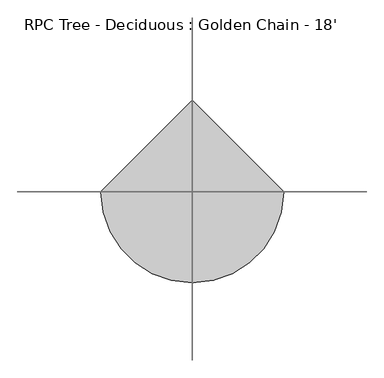
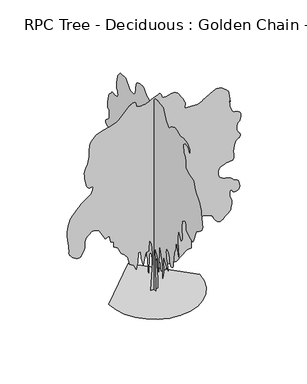
"""IFC4 building model written with IfcOpenShell, lengths in millimetres: geographic element geometry, RPC Tree - Deciduous : Golden Chain - 18'."""

from ifc_helpers import new_model, si_unit, origin, place, context, project, spatial, triangles, source, transform, mapped, element, save


def rpc_tree_deciduous_golden_chain_18_92130817(model_context):
    return source(origin(), model_context, "Body", "Tessellation", [
        triangles([(-0.0021439, 84.0442886, 0.0017013), (-0.0021439, -79.514705, 0.0017013), (-0.0021439, -54.9808464, 768.7285137), (-0.0021439, -30.4472354, 1202.1592524), (-0.0021439, -128.5824313, 1087.6687117), (-0.0021439, -161.2943336, 981.3544888), (-0.0021439, -161.2943336, 776.9073023), (-0.0021439, -202.1840252, 613.3465736), (-0.0021439, -226.7178838, 1406.6089096), (-0.0021439, -292.140671, 1251.2269695), (-0.0021439, -390.2761053, 932.2867716), (-0.0021439, -406.6337188, 556.102575), (-0.0021439, -447.5226474, 752.37348), (-0.0021439, -422.9887888, 1120.3813951), (-0.0021439, -398.4548939, 1226.6931473), (-0.0021439, -562.0131517, 1022.2459608), (-0.0021439, -643.7935524, 907.7528767), (-0.0021439, -570.1919403, 1161.2703238), (-0.0021439, -564.9696937, 1199.7284414), (-0.0021439, -559.9633495, 1237.6125389), (-0.0021439, -555.386267, 1274.3536102), (-0.0021439, -551.4518414, 1309.3777805), (-0.0021439, -548.3758664, 1342.1157532), (-0.0021439, -546.37181, 1371.9887844), (-0.0021439, -545.6580817, 1398.4301937), (-0.0021439, -546.8493608, 1421.534016), (-0.0021439, -550.1869114, 1442.0622688), (-0.0021439, -555.312616, 1460.4442863), (-0.0021439, -561.8709002, 1477.1091122), (-0.0021439, -569.5010668, 1492.488842), (-0.0021439, -577.8449615, 1507.0100487), (-0.0021439, -586.5470103, 1521.0994503), (-0.0021439, -614.3955648, 1489.5551548), (-0.0021439, -641.0985861, 1458.0134754), (-0.0021439, -665.5130842, 1426.4691799), (-0.0021439, -686.4960331, 1394.9248844), (-0.0021439, -702.8993196, 1363.383205), (-0.0021439, -713.5800631, 1331.8389095), (-0.0021439, -717.3950918, 1300.294614), (-0.0021439, -719.0638853, 1269.9442863), (-0.0021439, -723.7375099, 1241.7375778), (-0.0021439, -730.9130167, 1215.3215303), (-0.0021439, -740.0925436, 1190.333012), (-0.0021439, -750.773287, 1166.4189194), (-0.0021439, -762.4572395, 1143.2210621), (-0.0021439, -774.6391268, 1120.3813951), (-0.0021439, -797.2654346, 1120.6430071), (-0.0021439, -818.9620754, 1122.4794502), (-0.0021439, -838.7995274, 1127.4629396), (-0.0021439, -855.847978, 1137.1656904), (-0.0021439, -869.1753622, 1153.1626064), (-0.0021439, -877.8545563, 1177.0309896), (-0.0021439, -880.9533497, 1210.3380409), (-0.0021439, -882.6221432, 1252.4664288), (-0.0021439, -887.2956951, 1301.0338131), (-0.0021439, -894.4712019, 1354.9656956), (-0.0021439, -903.6508015, 1413.1900486), (-0.0021439, -914.3314722, 1474.6301937), (-0.0021439, -926.0154974, 1538.2190449), (-0.0021439, -938.1998554, 1602.8797783), (-0.0021439, -1003.6226789, 1758.2592476), (-0.0021439, -1028.1565012, 2036.3105896), (-0.0021439, -1134.4707968, 1611.0560234), (-0.0021439, -1093.5793247, 2028.1317284), (-0.0021439, -1118.113147, 2379.7846825), (-0.0021439, -1257.140126, 2134.4460239), (-0.0021439, -1267.5820759, 2148.5354256), (-0.0021439, -1277.5946915, 2163.0564869), (-0.0021439, -1286.7514, 2178.433746), (-0.0021439, -1294.6202511, 2195.1011879), (-0.0021439, -1300.7697304, 2213.4832054), (-0.0021439, -1304.7752998, 2234.0114582), (-0.0021439, -1306.2077705, 2257.1152805), (-0.0021439, -1304.3942184, 2284.415213), (-0.0021439, -1299.7206665, 2316.2921917), (-0.0021439, -1293.332539, 2351.3162167), (-0.0021439, -1286.3704639, 2388.0574333), (-0.0021439, -1279.9797203, 2425.0855511), (-0.0021439, -1275.3061684, 2460.9680992), (-0.0021439, -1273.4950871, 2494.2750778), (-0.0021439, -1274.6864388, 2526.5329926), (-0.0021439, -1278.0264965, 2560.0917), (-0.0021439, -1283.1522011, 2594.7116798), (-0.0021439, -1289.7079056, 2630.1702713), (-0.0021439, -1297.3381084, 2666.2889969), (-0.0021439, -1305.6820759, 2702.8396729), (-0.0021439, -1314.3840157, 2739.6188232), (-0.0021439, -1345.7607342, 2756.763707), (-0.0021439, -1376.1364964, 2771.6226837), (-0.0021439, -1404.5083111, 2781.8845573), (-0.0021439, -1429.8778381, 2785.2881287), (-0.0021439, -1451.239325, 2779.5474907), (-0.0021439, -1467.5969021, 2762.351738), (-0.0021439, -1477.9423462, 2731.439962), (-0.0021439, -1480.7337456, 2695.2194984), (-0.0021439, -1478.2292473, 2663.0124527), (-0.0021439, -1475.1534176, 2633.802317), (-0.0021439, -1476.2277706, 2606.5990356), (-0.0021439, -1486.169315, 2580.3861008), (-0.0021439, -1509.7024715, 2554.1987457), (-0.0021439, -1551.5464291, 2526.9879066), (-0.0021439, -1602.9255604, 2498.8777039), (-0.0021439, -1651.1601162, 2472.3397888), (-0.0021439, -1695.0995853, 2449.9522018), (-0.0021439, -1733.6059559, 2434.2878963), (-0.0021439, -1765.5313328, 2427.9227325), (-0.0021439, -1789.7298557, 2433.4293732), (-0.0021439, -1805.0613327, 2453.3862946), (-0.0021439, -1952.2644115, 2813.2027039), (-0.0021439, -2091.2889198, 2911.3481667), (-0.0021439, -2128.6269024, 2939.9231667), (-0.0021439, -2162.6730801, 2969.615831), (-0.0021439, -2192.1420662, 3000.6293449), (-0.0021439, -2215.746294, 3033.039576), (-0.0021439, -2232.1979061, 3067.0502907), (-0.0021439, -2240.209045, 3102.7626457), (-0.0021439, -2238.4919987, 3140.329248), (-0.0021439, -2229.7188423, 3187.039769), (-0.0021439, -2218.3701164, 3246.6282829), (-0.0021439, -2205.8758209, 3313.9381279), (-0.0021439, -2193.6685719, 3383.8138046), (-0.0021439, -2183.1783691, 3451.1236496), (-0.0021439, -2175.835358, 3510.7121635), (-0.0021439, -2173.0692478, 3557.3973953), (-0.0021439, -2164.9616032, 3599.7645767), (-0.0021439, -2142.2641514, 3649.0150589), (-0.0021439, -2107.4077034, 3703.9553101), (-0.0021439, -2062.820454, 3763.492955), (-0.0021439, -2010.9410625, 3826.4594604), (-0.0021439, -1954.194817, 3891.7374527), (-0.0021439, -1895.0179058, 3958.1331093), (-0.0021439, -1837.7740162, 4187.1141907), (-0.0021439, -1625.145425, 4236.1870674), (-0.0021439, -1453.4109947, 4317.9495186), (-0.0021439, -1454.7444889, 4324.4773178), (-0.0021439, -1458.0820759, 4341.9779938), (-0.0021439, -1462.4229446, 4367.5302132), (-0.0021439, -1466.7611973, 4398.0611984), (-0.0021439, -1470.0987843, 4430.6240364), (-0.0021439, -1471.4347492, 4462.1453682), (-0.0021439, -1469.7661011, 4489.7044418), (-0.0021439, -1464.1145565, 4515.6630318), (-0.0021439, -1454.6022011, 4544.1874535), (-0.0021439, -1441.8692574, 4574.8704643), (-0.0021439, -1426.5632149, 4607.280986), (-0.0021439, -1409.3241508, 4640.9614883), (-0.0021439, -1390.7999908, 4675.5308899), (-0.0021439, -1371.6305214, 4710.506662), (-0.0021439, -1338.9179832, 4906.7725891), (-0.0021439, -1445.2321335, 4996.7391907), (-0.0021439, -1576.0802513, 4972.2028976), (-0.0021439, -1649.6793926, 4865.8782829), (-0.0021439, -1649.6793926, 4964.0237457), (-0.0021439, -1535.1888519, 5070.3230713), (-0.0021439, -1347.0966991, 5094.8593643), (-0.0021439, -1199.8935476, 5062.1439194), (-0.0021439, -1052.6903961, 5143.9319504), (-0.0021439, -946.3761005, 5152.1111023), (-0.0021439, -938.5555023, 5148.3770279), (-0.0021439, -917.8620707, 5138.3694992), (-0.0021439, -888.4387213, 5123.7901566), (-0.0021439, -854.4407965, 5106.3400589), (-0.0021439, -820.0111393, 5087.7220093), (-0.0021439, -789.3025486, 5069.7132248), (-0.0021439, -766.462809, 5053.9653488), (-0.0021439, -750.6792521, 5038.3697891), (-0.0021439, -737.326506, 5021.3516418), (-0.0021439, -724.8322105, 5005.4770294), (-0.0021439, -711.6242231, 4993.3103302), (-0.0021439, -696.1277126, 4987.4426651), (-0.0021439, -676.7678478, 4990.465155), (-0.0021439, -651.9697975, 5004.8927628), (-0.0021439, -625.6020756, 5027.117569), (-0.0021439, -602.236605, 5051.5015457), (-0.0021439, -581.3730165, 5077.6383224), (-0.0021439, -562.5135209, 5105.2226852), (-0.0021439, -545.1577126, 5133.8994232), (-0.0021439, -528.8000991, 5163.2615845), (-0.0021439, -512.9454346, 5193.0051178), (-0.0021439, -414.8099639, 5397.4496155), (-0.0021439, -169.4723773, 5438.343631), (-0.0021439, -163.4401146, 5438.1913147), (-0.0021439, -147.2511773, 5437.2006775), (-0.0021439, -123.7660828, 5434.4828201), (-0.0021439, -95.8466569, 5429.1744232), (-0.0021439, -66.3536942, 5420.4621643), (-0.0021439, -38.1480076, 5407.4315643), (-0.0021439, -14.0911332, 5389.2710449), (-0.0021439, 3.3375856, 5370.932048), (-0.0021439, 15.1871941, 5356.7590759), (-0.0021439, 23.8896415, 5344.846431), (-0.0021439, 31.8767493, 5333.3907349), (-0.0021439, 41.5805652, 5320.4874527), (-0.0021439, 55.4332171, 5304.2826279), (-0.0021439, 75.8662495, 5282.9461395), (-0.0021439, 96.8951667, 5258.2575302), (-0.0021439, 112.9172356, 5234.5595581), (-0.0021439, 126.936765, 5213.8584961), (-0.0021439, 141.9573053, 5198.1611984), (-0.0021439, 160.9836875, 5189.5000992), (-0.0021439, 187.019453, 5189.8297302), (-0.0021439, 223.0691603, 5201.1836884), (-0.0021439, 263.6977487, 5220.8435349), (-0.0021439, 301.7494776, 5244.3891907), (-0.0021439, 337.654935, 5271.1352325), (-0.0021439, 371.8458713, 5300.4468155), (-0.0021439, 404.7490228, 5331.7146744), (-0.0021439, 436.7936874, 5364.2516418), (-0.0021439, 468.4065107, 5397.4496155), (-0.0021439, 491.2487575, 5406.0857162), (-0.0021439, 514.4465784, 5413.9090759), (-0.0021439, 538.360671, 5420.1825302), (-0.0021439, 563.3491894, 5424.0945007), (-0.0021439, 589.7652005, 5424.8560822), (-0.0021439, 617.9718727, 5421.6812759), (-0.0021439, 648.3223457, 5413.807338), (-0.0021439, 679.72181, 5404.5108124), (-0.0021439, 710.2653671, 5396.4845581), (-0.0021439, 739.0892618, 5388.0513519), (-0.0021439, 765.3401304, 5377.4595566), (-0.0021439, 788.156979, 5363.0069504), (-0.0021439, 806.6837551, 5342.991893), (-0.0021439, 820.0593922, 5315.6615845), (-0.0021439, 829.6199278, 5284.3687271), (-0.0021439, 837.4634897, 5253.4822403), (-0.0021439, 843.8769791, 5222.9771255), (-0.0021439, 849.1474422, 5192.7254837), (-0.0021439, 853.5569115, 5162.7284775), (-0.0021439, 857.3973747, 5132.8326279), (-0.0021439, 860.9483208, 5103.0379349), (-0.0021439, 866.3610718, 5073.4217194), (-0.0021439, 872.7034172, 5044.897879), (-0.0021439, 880.9050968, 5018.507048), (-0.0021439, 891.895705, 4995.3166031), (-0.0021439, 906.6073797, 4976.4444992), (-0.0021439, 925.9672445, 4962.9063721), (-0.0021439, 950.90751, 4955.8451752), (-0.0021439, 981.1385862, 4952.5180527), (-0.0021439, 1014.5192522, 4950.3588821), (-0.0021439, 1049.1851595, 4950.4606201), (-0.0021439, 1083.27959, 4954.016217), (-0.0021439, 1114.9432823, 4962.1442093), (-0.0021439, 1142.314286, 4976.0125488), (-0.0021439, 1163.533485, 4996.7391907), (-0.0021439, 1185.0142233, 5025.1618744), (-0.0021439, 1212.2201935, 5059.0452713), (-0.0021439, 1241.8544312, 5094.7832062), (-0.0021439, 1270.6326164, 5128.8195007), (-0.0021439, 1295.2629444, 5157.546817), (-0.0021439, 1312.4536102, 5177.4095581), (-0.0021439, 1318.9129543, 5184.8259659), (-0.0021439, 1572.4303288, 5168.4688248), (-0.0021439, 1670.5657631, 5045.7867783), (-0.0021439, 1675.8337555, 5036.8204651), (-0.0021439, 1681.1752899, 5026.6606201), (-0.0021439, 1686.6592575, 5014.0363907), (-0.0021439, 1692.3589096, 4997.7804062), (-0.0021439, 1698.3406666, 4976.6479752), (-0.0021439, 1704.683012, 4949.4444031), (-0.0021439, 1711.4546917, 4914.9511597), (-0.0021439, 1717.9875778, 4876.8767395), (-0.0021439, 1723.6619408, 4839.6656387), (-0.0021439, 1728.6225391, 4803.1402519), (-0.0021439, 1733.00919, 4767.2247116), (-0.0021439, 1736.9665066, 4731.7155418), (-0.0021439, 1740.6392475, 4696.5112953), (-0.0021439, 1744.1673752, 4661.4337852), (-0.0021439, 1726.808987, 4636.8466232), (-0.0021439, 1710.4538807, 4611.9798271), (-0.0021439, 1696.1003963, 4586.5546349), (-0.0021439, 1684.7516705, 4560.2402527), (-0.0021439, 1677.408514, 4532.8082062), (-0.0021439, 1675.0717381, 4503.9282829), (-0.0021439, 1678.7446243, 4473.3467194), (-0.0021439, 1687.7336105, 4446.5242287), (-0.0021439, 1700.5834076, 4427.9823372), (-0.0021439, 1717.1544891, 4416.0444031), (-0.0021439, 1737.3016605, 4408.9576263), (-0.0021439, 1760.8805992, 4405.0206573), (-0.0021439, 1787.7511974, 4402.5315651), (-0.0021439, 1817.7689873, 4399.7375496), (-0.0021439, 1846.9991798, 4399.6105225), (-0.0021439, 1872.3687069, 4403.8015457), (-0.0021439, 1895.0179058, 4408.5259666), (-0.0021439, 1916.094817, 4410.1261597), (-0.0021439, 1936.7425392, 4404.8683411), (-0.0021439, 1958.1038807, 4389.0187271), (-0.0021439, 1981.3271725, 4358.8435341), (-0.0021439, 2004.8831474, 4328.2872597), (-0.0021439, 2026.5797882, 4309.5930519), (-0.0021439, 2046.5593826, 4296.6136116), (-0.0021439, 2064.9668346, 4283.2278008), (-0.0021439, 2081.9416706, 4263.2380325), (-0.0021439, 2097.6312653, 4230.5228783), (-0.0021439, 2112.1752903, 4178.9353294), (-0.0021439, 2125.1928097, 4121.9123566), (-0.0021439, 2136.208707, 4075.3541519), (-0.0021439, 2145.220657, 4036.6698853), (-0.0021439, 2152.2311302, 4003.269017), (-0.0021439, 2157.2373653, 3972.5857155), (-0.0021439, 2160.239653, 3942.0294411), (-0.0021439, 2161.2429348, 3909.0602325), (-0.0021439, 2158.6191124, 3878.529538), (-0.0021439, 2151.2761013, 3856.1774139), (-0.0021439, 2139.9984467, 3840.6074341), (-0.0021439, 2125.5737457, 3830.4725876), (-0.0021439, 2108.7894505, 3824.4276077), (-0.0021439, 2090.4303967, 3821.0746147), (-0.0021439, 2071.2837456, 3819.093631), (-0.0021439, 2071.2837456, 3606.4699814), (-0.0021439, 2071.4514679, 3602.8379356), (-0.0021439, 2072.6198559, 3598.3167), (-0.0021439, 2075.7897205, 3592.093824), (-0.0021439, 2081.9671051, 3583.305407), (-0.0021439, 2092.1472977, 3571.0625496), (-0.0021439, 2107.334016, 3554.5525108), (-0.0021439, 2128.5303967, 3532.8863914), (-0.0021439, 2153.3512653, 3510.1278969), (-0.0021439, 2177.8850876, 3490.1125488), (-0.0021439, 2200.8441513, 3471.4944992), (-0.0021439, 2220.9432152, 3453.054055), (-0.0021439, 2236.8944218, 3433.4453682), (-0.0021439, 2247.4099136, 3411.4234566), (-0.0021439, 2251.1996532, 3385.6677612), (-0.0021439, 2244.7632729, 3361.4363914), (-0.0021439, 2226.7369022, 3344.0880318), (-0.0021439, 2199.0560337, 3332.4547302), (-0.0021439, 2163.6509274, 3325.3935333), (-0.0021439, 2122.4495178, 3321.7614876), (-0.0021439, 2077.3874428, 3320.440638), (-0.0021439, 2030.394817, 3320.2374527), (-0.0021439, 2016.5671726, 3321.7614876), (-0.0021439, 2003.8823364, 3321.9393837), (-0.0021439, 1993.4861687, 3319.3991318), (-0.0021439, 1986.5265644, 3312.7698853), (-0.0021439, 1984.1415356, 3300.704924), (-0.0021439, 1987.4789772, 3281.8325294), (-0.0021439, 1997.6847496, 3254.8324333), (-0.0021439, 2015.3987846, 3226.9687271), (-0.0021439, 2039.2646244, 3205.2770279), (-0.0021439, 2067.4229347, 3187.8780899), (-0.0021439, 2098.0122013, 3172.892086), (-0.0021439, 2129.1729446, 3158.4903488), (-0.0021439, 2159.0484467, 3142.8183403), (-0.0021439, 2185.7769024, 3123.9715256), (-0.0021439, 2209.1905895, 3107.7664101), (-0.0021439, 2229.8839485, 3098.4193062), (-0.0021439, 2247.1458309, 3091.789769), (-0.0021439, 2260.259856, 3083.7379349), (-0.0021439, 2268.5097885, 3070.0983604), (-0.0021439, 2271.1792477, 3046.7303101), (-0.0021439, 2267.5547596, 3009.4939201), (-0.0021439, 2258.1617283, 2968.2188232), (-0.0021439, 2244.4762264, 2934.6653481), (-0.0021439, 2227.2144894, 2907.5635139), (-0.0021439, 2207.0926071, 2885.592762), (-0.0021439, 2184.8218735, 2867.5078194), (-0.0021439, 2161.1236107, 2851.9884178), (-0.0021439, 2136.7091125, 2837.7389969), (-0.0021439, 2128.1010624, 2820.1877426), (-0.0021439, 2120.4252228, 2802.3315651), (-0.0021439, 2114.6061012, 2783.8911209), (-0.0021439, 2111.5783791, 2764.6123558), (-0.0021439, 2112.2691799, 2744.1653481), (-0.0021439, 2117.6108597, 2722.2960434), (-0.0021439, 2128.5303967, 2698.7248077), (-0.0021439, 2148.3677032, 2676.3473946), (-0.0021439, 2177.0748173, 2656.8148659), (-0.0021439, 2210.5012653, 2637.9933403), (-0.0021439, 2244.4991901, 2617.7495178), (-0.0021439, 2274.9232052, 2593.9245186), (-0.0021439, 2297.620657, 2564.3841705), (-0.0021439, 2308.446159, 2526.9879066), (-0.0021439, 2310.9024044, 2485.6212456), (-0.0021439, 2311.0675106, 2444.3970177), (-0.0021439, 2308.6595181, 2401.4558887), (-0.0021439, 2303.3915257, 2354.9408501), (-0.0021439, 2294.9740162, 2302.9877712), (-0.0021439, 2283.1248848, 2243.7396435), (-0.0021439, 2267.5547596, 2175.3349525), (-0.0021439, 2251.3672302, 2117.0648174), (-0.0021439, 2237.1813229, 2082.6833405), (-0.0021439, 2223.9962265, 2062.0356182), (-0.0021439, 2210.8111301, 2044.9642765), (-0.0021439, 2196.6252228, 2021.3144119), (-0.0021439, 2180.4352226, 1980.9232727), (-0.0021439, 2161.2429348, 1913.6411877), (-0.0021439, 2144.2656281, 1837.9644115), (-0.0021439, 2133.5848846, 1778.8840061), (-0.0021439, 2126.4805218, 1735.9681664), (-0.0021439, 2120.2346821, 1708.7877033), (-0.0021439, 2112.1270374, 1696.9131374), (-0.0021439, 2099.4422012, 1699.9180412), (-0.0021439, 2079.4626068, 1717.370319), (-0.0021439, 2055.4062263, 1753.7304543), (-0.0021439, 2032.2085144, 1808.9728672), (-0.0021439, 2009.7244217, 1875.9475582), (-0.0021439, 1987.8118057, 1947.4968246), (-0.0021439, 1966.3309948, 2016.4731377), (-0.0021439, 1945.1347595, 2075.7211201), (-0.0021439, 1924.0831375, 2118.0884468), (-0.0021439, 1898.5232151, 2149.1551552), (-0.0021439, 1864.8097206, 2179.3659565), (-0.0021439, 1824.3018734, 2208.8579063), (-0.0021439, 1778.3583115, 2237.7782341), (-0.0021439, 1728.3354927, 2266.2695183), (-0.0021439, 1675.5974327, 2294.4762268), (-0.0021439, 1621.4979733, 2322.5380314), (-0.0021439, 1576.1971046, 2351.8395859), (-0.0021439, 1532.4709946, 2378.2097786), (-0.0021439, 1491.8919308, 2398.715213), (-0.0021439, 1456.032201, 2410.4220566), (-0.0021439, 1426.4667091, 2410.3966221), (-0.0021439, 1404.769923, 2395.7104546), (-0.0021439, 1392.5144211, 2363.42696), (-0.0021439, 1384.3127415, 2321.608437), (-0.0021439, 1373.9674427, 2280.2191029), (-0.0021439, 1361.8312649, 2239.1854156), (-0.0021439, 1348.2650871, 2198.4387749), (-0.0021439, 1333.6245564, 2157.9054932), (-0.0021439, 1318.270261, 2117.5168247), (-0.0021439, 1302.557848, 2077.1995182), (-0.0021439, 1122.642013, 1921.8200489), (-0.0021439, 1105.2379154, 1902.4119312), (-0.0021439, 1088.5475824, 1882.2163616), (-0.0021439, 1073.2897928, 1860.4485043), (-0.0021439, 1060.1757677, 1836.3210526), (-0.0021439, 1049.9243586, 1809.0440838), (-0.0021439, 1043.2491846, 1777.8350876), (-0.0021439, 1040.8641558, 1741.9041412), (-0.0021439, 1040.1478477, 1706.9283691), (-0.0021439, 1038.1463711, 1678.3863613), (-0.0021439, 1035.070396, 1655.2139385), (-0.0021439, 1031.1359705, 1636.3290447), (-0.0021439, 1026.5588516, 1620.6648846), (-0.0021439, 1021.5525438, 1607.1469597), (-0.0021439, 1016.3302608, 1594.7010624), (-0.0021439, 869.1271093, 1496.5656281), (-0.0021439, 852.7720757, 1324.8285816), (-0.0021439, 730.1027464, 1267.5820759), (-0.0021439, 697.3900629, 1054.9560282), (-0.0021439, 566.5419814, 1022.2459608), (-0.0021439, 578.5586898, 1016.8332098), (-0.0021439, 589.0742907, 1010.4907917), (-0.0021439, 596.5850967, 1002.2891848), (-0.0021439, 599.5873844, 991.2985765), (-0.0021439, 596.5850967, 976.5869019), (-0.0021439, 586.0694959, 957.227037), (-0.0021439, 566.5419814, 932.2867716), (-0.0021439, 542.9631517, 906.6327415), (-0.0021439, 521.098825, 885.268784), (-0.0021439, 500.6670779, 867.4837503), (-0.0021439, 481.3782844, 852.5587166), (-0.0021439, 462.9480503, 839.7799181), (-0.0021439, 445.0893293, 828.4287214), (-0.0021439, 427.5175821, 817.7962309), (-0.0021439, 415.2874784, 850.3895176), (-0.0021439, 403.27077, 878.7613323), (-0.0021439, 391.6832869, 898.6927465), (-0.0021439, 380.7384244, 905.9647591), (-0.0021439, 370.6545922, 896.3558979), (-0.0021439, 361.6401352, 865.6473072), (-0.0021439, 353.9160064, 809.6174423), (-0.0021439, 346.4306348, 755.6856325), (-0.0021439, 338.0841966, 726.6457626), (-0.0021439, 329.0239938, 711.3397928), (-0.0021439, 319.3923142, 698.6092472), (-0.0021439, 309.3313731, 677.2936152), (-0.0021439, 298.9834219, 636.2370369), (-0.0021439, 288.4932192, 564.2788201), (-0.0021439, 279.4076364, 484.1215035), (-0.0021439, 272.9001666, 423.7050605), (-0.0021439, 268.5364431, 379.7401932), (-0.0021439, 265.889766, 348.9350604), (-0.0021439, 264.5308555, 328.0029442), (-0.0021439, 264.0304863, 313.6493872), (-0.0021439, 263.9593606, 302.5851461), (-0.0021439, 239.4252477, 809.6174423), (-0.0021439, 227.0988743, 842.5688467), (-0.0021439, 214.4146195, 873.4450871), (-0.0021439, 201.0151103, 900.1709993), (-0.0021439, 186.5429559, 920.6764338), (-0.0021439, 170.6400022, 932.8836828), (-0.0021439, 152.9489127, 934.7200533), (-0.0021439, 133.1120149, 924.1105265), (-0.0021439, 115.4209072, 902.0556953), (-0.0021439, 103.7379267, 871.8474375), (-0.0021439, 97.0620442, 834.8447542), (-0.0021439, 94.3917403, 792.4038855), (-0.0021439, 94.7254953, 745.8888468), (-0.0021439, 97.0620442, 696.65348), (-0.0021439, 100.3998583, 646.0591845), (-0.0021439, 84.0442886, 237.1621046), (88.2248747, 0.0002499, 0.0), (-86.1796688, 0.0002499, 0.0), (-44.6549823, 0.000202, 805.5838949), (-36.3499433, 0.0001914, 1029.8176643), (-69.5698451, 0.0001754, 1303.8836391), (-127.7051138, 0.0001648, 1445.0670273), (-144.3149375, 0.0001861, 1137.7829493), (-227.3643014, 0.0001861, 1112.8680456), (-293.8043594, 0.000202, 797.2781519), (-351.9398915, 0.0001914, 996.5995611), (-360.2456709, 0.0001808, 1179.3068682), (-426.6844571, 0.0001808, 1179.3068682), (-443.2935451, 0.0001967, 913.5491798), (-484.8200074, 0.0002073, 730.8393293), (-551.2587936, 0.000202, 872.0227175), (-659.2240059, 0.0001967, 938.4640108), (-700.7479248, 0.0001808, 1154.3919645), (-783.7983788, 0.0001754, 1254.0539772), (-875.1545031, 0.0001754, 1328.7985428), (-974.8139723, 0.0001595, 1519.8115929), (-1082.7792572, 0.0001595, 1577.9471432), (-1082.7792572, 0.0001489, 1719.1331474), (-1157.5238228, 0.0001489, 1744.0479057), (-1199.0477417, 0.0001382, 1935.0611012), (-1315.3188423, 0.0001382, 1885.2312939), (-1464.8079735, 0.0001223, 2167.6005409), (-1498.6102707, 0.0001223, 2188.6191708), (-1532.3364098, 0.0001223, 2207.6005703), (-1565.920261, 0.000117, 2222.5153576), (-1599.2856663, 0.000117, 2231.3292091), (-1632.3590836, 0.000117, 2232.0073654), (-1665.071767, 0.000117, 2222.5153576), (-1697.3475586, 0.0001223, 2200.8213329), (-1729.1864582, 0.0001223, 2173.6305508), (-1759.8645275, 0.0001223, 2148.0374908), (-1788.2186108, 0.0001276, 2122.5893349), (-1813.0851162, 0.0001276, 2095.8354446), (-1833.3035042, 0.0001276, 2066.3206764), (-1847.7078575, 0.0001329, 2032.5919212), (-1855.1424328, 0.0001329, 1993.1966515), (-1857.4665642, 0.0001382, 1950.0978287), (-1858.4826359, 0.0001382, 1906.709634), (-1859.9354542, 0.0001435, 1863.7555698), (-1863.5676453, 0.0001435, 1821.9649521), (-1871.12169, 0.0001435, 1782.0615738), (-1884.3423946, 0.0001489, 1744.7744602), (-1904.9722401, 0.0001489, 1710.8272591), (-1925.8916027, 0.0001542, 1679.5447208), (-1941.1469215, 0.0001542, 1650.7309273), (-1954.2202515, 0.0001542, 1625.8414581), (-1968.6042572, 0.0001542, 1606.3240448), (-1987.7812843, 0.0001595, 1593.6367378), (-2015.2387653, 0.0001595, 1589.2298847), (-2054.4613712, 0.0001595, 1594.5563038), (-2100.8772881, 0.0001542, 1610.4896336), (-2146.1325199, 0.0001542, 1635.5747303), (-2188.0426071, 0.0001542, 1667.7768345), (-2224.4355892, 0.0001489, 1705.0640934), (-2253.1274426, 0.0001489, 1745.4043636), (-2271.9412651, 0.0001435, 1786.7580894), (-2278.6952133, 0.0001435, 1827.0983597), (-2278.3572979, 0.0001435, 1862.6177032), (-2278.0195278, 0.0001382, 1894.6496143), (-2278.6952133, 0.0001382, 1928.8635143), (-2281.4078384, 0.0001329, 1970.9208309), (-2287.1711494, 0.0001329, 2026.4883694), (-2297.0009274, 0.0001276, 2101.2355511), (-2311.91586, 0.0001223, 2200.8213329), (-2322.6194218, 0.0001116, 2312.733688), (-2321.2629639, 0.0001063, 2418.8346245), (-2311.0445469, 0.000101, 2516.3629738), (-2295.1619408, 9.57e-05, 2602.5603287), (-2276.8079739, 9.04e-05, 2674.6710434), (-2259.1802708, 9.04e-05, 2729.9159271), (-2245.4770374, 8.51e-05, 2765.552124), (-2223.2494698, 8.51e-05, 2800.0962364), (-2182.5714294, 7.97e-05, 2849.5754837), (-2130.4174908, 7.97e-05, 2907.6399628), (-2073.7603386, 7.44e-05, 2967.8886108), (-2019.5719311, 7.44e-05, 3023.9209465), (-1974.8248077, 6.91e-05, 3069.3361977), (-1946.496159, 6.91e-05, 3097.7588814), (-1919.5238228, 6.38e-05, 3119.3488426), (-1878.1676262, 6.38e-05, 3147.4921829), (-1828.3860718, 6.38e-05, 3180.5628387), (-1776.1357727, 5.85e-05, 3216.9864876), (-1727.37029, 5.85e-05, 3255.1373566), (-1688.0485622, 5.32e-05, 3293.4405418), (-1664.1269119, 5.32e-05, 3330.2958504), (-1652.0695084, 5.32e-05, 3362.9857155), (-1643.9338131, 4.78e-05, 3390.4430511), (-1639.0672497, 4.78e-05, 3413.5317581), (-1636.8141895, 4.78e-05, 3433.1657341), (-1636.5246723, 4.78e-05, 3450.1585922), (-1637.5405987, 4.78e-05, 3465.3983597), (-1639.2120083, 4.25e-05, 3479.8003876), (-1669.3566799, 4.25e-05, 3474.8727814), (-1698.8486298, 4.25e-05, 3472.5104256), (-1727.0325199, 4.25e-05, 3475.2029938), (-1753.2554832, 4.25e-05, 3485.5407349), (-1776.8621819, 4.25e-05, 3506.0639008), (-1797.2025101, 4.25e-05, 3539.2871635), (-1813.6185139, 3.72e-05, 3587.7501938), (-1828.0965546, 3.19e-05, 3649.192955), (-1841.9954155, 3.19e-05, 3717.1379356), (-1853.7124329, 2.66e-05, 3788.029248), (-1861.6551167, 2.13e-05, 3858.1586884), (-1864.2229832, 1.59e-05, 3923.9447891), (-1859.8161301, 1.59e-05, 3981.7552139), (-1846.8366898, 1.06e-05, 4027.907048), (-1827.3218925, 1.06e-05, 4070.527993), (-1805.6277225, 5.3e-06, 4119.6770279), (-1783.6414192, 5.3e-06, 4174.7951752), (-1763.2554543, 0.0, 4235.2725883), (-1746.3543056, -5.3e-06, 4300.5505806), (-1734.827829, -1.06e-05, 4370.0448853), (-1730.5682053, -1.06e-05, 4443.1715263), (-1731.1981087, -1.59e-05, 4512.6914108), (-1731.5358788, -2.13e-05, 4573.1941132), (-1729.2601456, -2.13e-05, 4626.8643837), (-1722.0438709, -2.66e-05, 4675.9116806), (-1707.5659756, -3.19e-05, 4722.4698853), (-1683.4969505, -3.19e-05, 4768.7234573), (-1647.5177513, -3.72e-05, 4816.881855), (-1600.690377, -3.72e-05, 4863.1860054), (-1547.4697884, -4.25e-05, 4902.5054077), (-1490.6194794, -4.25e-05, 4934.9917969), (-1432.8953865, -4.25e-05, 4960.8233597), (-1377.0611492, -4.25e-05, 4980.0768356), (-1325.8750294, -4.78e-05, 4992.9801178), (-1282.0980503, -4.78e-05, 4999.6093643), (-1235.7558208, -4.78e-05, 5007.4071442), (-1178.8064627, -4.78e-05, 5022.3172806), (-1116.9168537, -4.78e-05, 5042.3067581), (-1055.7561974, -4.78e-05, 5065.3698853), (-1000.9861393, -5.32e-05, 5089.4236496), (-958.2760283, -5.32e-05, 5112.4867767), (-933.2875099, -5.32e-05, 5132.4768356), (-667.5298216, -6.91e-05, 5414.8485535), (-644.4056517, -6.91e-05, 5430.6981674), (-621.3551691, -7.44e-05, 5445.4304077), (-598.4494452, -7.44e-05, 5458.0034775), (-575.7621672, -7.44e-05, 5467.2994217), (-553.3669862, -7.44e-05, 5472.2270279), (-531.3324663, -7.44e-05, 5471.7195007), (-509.7348747, -7.44e-05, 5464.6833023), (-494.6015325, -7.44e-05, 5448.9860046), (-488.3302946, -6.91e-05, 5425.5926651), (-485.5464529, -6.91e-05, 5398.0083023), (-480.8728283, -6.91e-05, 5369.6617767), (-468.9348215, -6.91e-05, 5344.109848), (-444.3603404, -6.38e-05, 5324.7802139), (-401.7696261, -6.38e-05, 5315.1790558), (-351.2845536, -6.38e-05, 5313.8076279), (-306.0319379, -6.38e-05, 5316.3475891), (-265.1379224, -6.38e-05, 5322.1640945), (-227.7280329, -6.38e-05, 5330.5967194), (-192.9340992, -6.38e-05, 5340.9856201), (-159.8838637, -6.91e-05, 5352.6692093), (-127.7051138, -6.91e-05, 5365.0138046), (-76.3011021, -6.91e-05, 5394.9858124), (-26.1320305, -6.91e-05, 5423.3067581), (21.5672178, -7.44e-05, 5448.2750015), (65.5619775, -7.44e-05, 5468.2139008), (104.6172789, -7.44e-05, 5481.4729752), (137.4980844, -7.44e-05, 5486.4005814), (162.9699762, -7.44e-05, 5481.295079), (179.3133463, -7.44e-05, 5468.6964294), (187.9572228, -7.44e-05, 5452.7706573), (192.3880025, -7.44e-05, 5434.2287659), (196.092591, -6.91e-05, 5413.7817581), (202.5574036, -6.91e-05, 5392.1917969), (215.2690732, -6.91e-05, 5370.1448868), (237.7143056, -6.91e-05, 5348.4020279), (275.0261451, -6.38e-05, 5338.7758713), (326.72021, -6.91e-05, 5346.5736511), (387.858048, -6.91e-05, 5362.8040558), (453.4992448, -6.91e-05, 5378.4251953), (518.703586, -6.91e-05, 5384.495755), (578.5332916, -6.91e-05, 5371.9482651), (628.0480745, -6.38e-05, 5331.7908325), (667.8549471, -6.38e-05, 5276.5453674), (702.431979, -5.85e-05, 5224.3485535), (732.6477945, -5.85e-05, 5174.6917007), (759.3787937, -5.32e-05, 5127.0667007), (783.4960716, -5.32e-05, 5080.9654449), (805.8683979, -4.78e-05, 5035.8804062), (827.3694838, -4.78e-05, 4991.303476), (819.0637407, -3.72e-05, 4841.7992294), (1101.4329878, -3.72e-05, 4825.1874527), (1128.1156614, -3.72e-05, 4827.1178581), (1154.7247204, -3.72e-05, 4829.8104263), (1181.1890207, -3.72e-05, 4834.1284767), (1207.4373459, -3.72e-05, 4840.8338814), (1233.3936104, -3.72e-05, 4850.7399628), (1258.9866703, -3.72e-05, 4864.6338821), (1284.1428383, -3.72e-05, 4883.3280899), (1314.3840157, -4.25e-05, 4906.391217), (1354.2163227, -4.25e-05, 4932.4774155), (1402.0343342, -4.25e-05, 4961.1285736), (1456.2481762, -4.78e-05, 4991.8115845), (1515.2548943, -4.78e-05, 5024.0189209), (1577.4569115, -4.78e-05, 5057.2168945), (1641.2566509, -5.32e-05, 5090.9479752), (1680.2888615, -5.32e-05, 5087.2394806), (1718.5920467, -5.32e-05, 5082.6676666), (1755.4448845, -5.32e-05, 5076.3680511), (1790.1184948, -4.78e-05, 5067.4273178), (1821.883707, -4.78e-05, 5055.0065643), (1850.0193443, -4.78e-05, 5038.2174728), (1873.796236, -4.78e-05, 5016.2211411), (1895.5158405, -4.78e-05, 4994.8090759), (1917.3800583, -4.25e-05, 4978.1972992), (1938.5180122, -4.25e-05, 4963.0331085), (1958.0582439, -4.25e-05, 4945.9899628), (1975.1269695, -4.25e-05, 4923.7139969), (1988.8557827, -3.72e-05, 4892.8786697), (1998.3730797, -3.72e-05, 4850.1051178), (2031.5912556, -2.13e-05, 4609.2622604), (2026.3130894, -2.66e-05, 4631.7411209), (2021.3982731, -2.66e-05, 4650.2068542), (2017.2097206, -2.66e-05, 4660.6972023), (2014.1109272, -2.66e-05, 4659.1984566), (2012.4624813, -2.66e-05, 4641.7233604), (2012.6326744, -2.13e-05, 4604.2584961), (2014.982095, -2.13e-05, 4542.8157349), (2024.0372108, -1.59e-05, 4472.7371635), (2041.6649139, -1.06e-05, 4412.2344612), (2064.2302517, -5.3e-06, 4361.7392876), (2088.1036491, -5.3e-06, 4321.7088821), (2109.6530605, -5.3e-06, 4292.6004845), (2125.2461494, -5.3e-06, 4274.7948853), (2131.2507248, 0.0, 4268.7751945), (2142.2438038, 0.0, 4269.5626465), (2170.3794411, 0.0, 4269.054538), (2208.3929638, 0.0, 4262.8822403), (2249.0228966, 0.0, 4246.6771248), (2285.0019505, 0.0, 4216.0955612), (2309.0709755, 5.3e-06, 4166.7686302), (2313.9605026, 1.06e-05, 4094.3532829), (2302.3145565, 1.06e-05, 4025.0874527), (2283.8411201, 1.59e-05, 3981.5264488), (2261.8803967, 1.59e-05, 3953.8150589), (2239.7721531, 1.59e-05, 3932.0472015), (2220.8644409, 2.13e-05, 3906.3423752), (2208.4894695, 2.13e-05, 3866.8453674), (2205.9977612, 2.66e-05, 3803.6756767), (2214.1080219, 2.66e-05, 3738.0166031), (2229.1931477, 3.19e-05, 3693.2617767), (2248.052607, 3.19e-05, 3662.9089783), (2267.4963329, 3.72e-05, 3640.404538), (2284.3237942, 3.72e-05, 3619.1700783), (2295.3423077, 3.72e-05, 3592.7539581), (2297.3514874, 4.25e-05, 3554.5272217), (2288.6113232, 4.25e-05, 3520.3133217), (2271.1538132, 4.25e-05, 3503.5492287), (2247.4479927, 4.25e-05, 3494.176545), (2219.9678387, 4.25e-05, 3482.1877419), (2191.1768635, 4.78e-05, 3457.5500015), (2163.5518055, 4.78e-05, 3410.2805031), (2139.5564678, 5.32e-05, 3330.2958504), (2124.616246, 5.85e-05, 3235.8585915), (2119.7039005, 6.38e-05, 3152.4703674), (2120.5978867, 6.91e-05, 3080.9947884), (2123.0922112, 7.44e-05, 3022.3207535), (2122.9702709, 7.44e-05, 2977.2865837), (2116.0208405, 7.44e-05, 2946.7811783), (2098.0325489, 7.97e-05, 2931.6681473), (2075.2233307, 7.97e-05, 2926.3088814), (2054.8856186, 7.97e-05, 2923.4387077), (2034.4005318, 7.97e-05, 2921.4065643), (2011.1568924, 7.97e-05, 2918.688707), (1982.5362556, 7.97e-05, 2913.6343643), (1945.927153, 7.97e-05, 2904.642762), (1898.7111397, 7.97e-05, 2890.1392868), (1848.9295853, 7.97e-05, 2873.0196922), (1806.557317, 7.97e-05, 2855.9000977), (1771.8863228, 8.51e-05, 2836.7483597), (1745.2036491, 8.51e-05, 2813.5329163), (1726.8014294, 8.51e-05, 2784.1957535), (1716.9715061, 9.04e-05, 2746.7561783), (1716.0038326, 9.04e-05, 2699.1311783), (1719.3693249, 9.57e-05, 2651.9381287), (1723.6059849, 9.57e-05, 2615.4889), (1730.6011974, 9.57e-05, 2587.3202705), (1742.2496143, 0.000101, 2564.9937263), (1760.4309174, 0.000101, 2545.9693062), (1787.0425198, 0.000101, 2527.8387268), (1823.9665741, 0.000101, 2508.1053383), (1868.3733112, 0.000101, 2489.8733116), (1914.8146626, 0.0001063, 2476.1444984), (1961.2535431, 0.0001063, 2464.3056862), (2005.6604256, 0.0001063, 2451.7378487), (2045.9980797, 0.0001063, 2435.8296627), (2080.234798, 0.0001063, 2413.9679157), (2106.3358212, 0.0001116, 2383.5311108), (2130.3794117, 0.0001116, 2355.9518349), (2158.3448559, 0.0001116, 2339.8507828), (2188.0552517, 0.0001116, 2328.3978481), (2217.3287556, 0.0001116, 2314.7681568), (2243.9859947, 0.000117, 2292.1266609), (2265.8503578, 0.000117, 2253.6532825), (2280.7423267, 0.0001223, 2192.5154446), (2284.6387459, 0.0001276, 2127.6997787), (2276.3354736, 0.0001276, 2080.7503189), (2257.8595665, 0.0001276, 2048.6929733), (2231.2504349, 0.0001329, 2028.5482727), (2198.5377514, 0.0001329, 2017.3367477), (2161.758601, 0.0001329, 2012.084016), (2122.9474525, 0.0001329, 2009.8056667), (2101.7129929, 0.0001329, 2041.1618923), (2081.2050877, 0.0001276, 2068.4491802), (2062.1473846, 0.0001276, 2087.6032436), (2045.2716705, 0.0001276, 2094.5502033), (2031.301593, 0.0001276, 2085.2283886), (2020.9613811, 0.0001276, 2055.5688618), (2014.982095, 0.0001329, 2001.5023945), (2017.3316608, 0.0001382, 1943.077327), (2028.6854736, 0.0001382, 1899.1784077), (2044.8347786, 0.0001435, 1863.9969795), (2061.5657341, 0.0001435, 1831.721188), (2074.6671146, 0.0001435, 1796.5396145), (2079.9198463, 0.0001489, 1752.6433113), (2073.1151745, 0.0001489, 1694.2182438), (2060.9612652, 0.0001542, 1634.6526936), (2051.1314873, 0.0001595, 1588.8921146), (2040.8648174, 0.0001595, 1553.4438423), (2027.4027031, 0.0001595, 1524.8256763), (2007.9844116, 0.0001648, 1499.5475681), (1979.8489197, 0.0001648, 1474.1220852), (1940.2375294, 0.0001648, 1445.0670273), (1897.6468151, 0.0001701, 1411.1936588), (1860.8676647, 0.0001701, 1376.4489773), (1827.5758015, 0.0001701, 1345.0443535), (1795.4449139, 0.0001754, 1321.1937744), (1762.1530506, 0.0001754, 1309.1135525), (1725.3739002, 0.0001754, 1313.0099716), (1682.783186, 0.0001701, 1337.101815), (1643.0500008, 0.0001701, 1374.8030022), (1614.0660141, 0.0001701, 1414.9706085), (1592.3464096, 0.0001648, 1454.995927), (1574.4063709, 0.0001648, 1492.2577515), (1556.7559948, 0.0001595, 1524.1473747), (1535.9077034, 0.0001595, 1548.0437359), (1508.376535, 0.0001595, 1561.3381279), (1468.1125683, 0.0001595, 1573.6367958), (1415.0620274, 0.0001595, 1592.6208115), (1354.7472496, 0.0001542, 1612.7655121), (1292.689991, 0.0001542, 1628.5516125), (1234.4096821, 0.0001542, 1634.4596821), (1185.4282242, 0.0001542, 1624.9676743), (1151.2627224, 0.0001595, 1594.5563038), (1124.6054106, 0.0001595, 1573.5402901), (1095.6214966, 0.0001595, 1585.0667667), (1066.0584028, 0.0001542, 1612.8620178), (1037.6561394, 0.0001542, 1640.6597397), (1012.1621286, 0.0001542, 1652.1837456), (991.3138372, 0.0001542, 1631.1678772), (976.8586876, 0.0001595, 1561.3381279), (969.4749086, 0.0001648, 1473.9062553), (967.6105602, 0.0001701, 1406.9568535), (969.6679201, 0.0001701, 1354.5363613), (974.0494114, 0.0001754, 1310.6858402), (979.1599279, 0.0001754, 1269.4514385), (983.3966606, 0.0001808, 1224.8769791), (985.1645033, 0.0001808, 1171.0035959), (993.4677755, 0.000202, 830.4987986), (868.8934027, 0.000202, 805.5838949), (727.7100872, 0.0002127, 689.312867), (586.5241556, 0.000218, 589.6534341), (395.5085258, 0.000218, 597.9592134), (329.0697395, 0.000218, 556.4352945), (304.1548722, 0.0002233, 456.7733182), (277.6423372, 0.0002233, 451.6907796), (252.2182168, 0.0002233, 448.1296961), (228.9739052, 0.0002233, 447.6216966), (208.9983258, 0.0002233, 451.6907796), (193.3811286, 0.0002233, 461.8584002), (183.2117457, 0.0002233, 479.6561874), (179.5797908, 0.0002233, 506.6030528), (179.4588861, 0.000218, 541.3019886), (178.6112816, 0.000218, 579.775367), (176.311313, 0.0002127, 619.7016363), (171.8320261, 0.0002127, 658.7566652), (164.4472298, 0.0002127, 694.616395), (153.4302423, 0.0002073, 724.9541508), (138.0551089, 0.0002073, 747.4484173), (121.4691572, 0.0002073, 766.2139143), (107.062533, 0.0002073, 786.7218922), (94.4717499, 0.000202, 808.682761), (83.3338487, 0.000202, 831.8068583), (73.2856112, 0.000202, 855.8022686), (63.9638101, 0.000202, 880.376786), (55.0049729, 0.0001967, 905.2433641), (63.3100119, 0.0002127, 689.312867), (88.2248747, 0.0002339, 265.7602136), (-1213.063456, 0.0, 0.0051038), (-1180.9933931, -277.9547636, 0.0051038), (-1089.6600872, -533.209532, 0.0051038), (-946.3761005, -758.4542135, 0.0051038), (-758.4542135, -946.3761005, 0.0051038), (-533.209532, -1089.6600872, 0.0051038), (-277.9547636, -1180.9933931, 0.0051038), (5.3e-05, -1213.063456, 0.0051038), (277.9547636, -1180.9933931, 0.0051038), (533.209532, -1089.6600872, 0.0051038), (758.4542135, -946.3761005, 0.0051038), (946.3761005, -758.4542135, 0.0051038), (1089.6600872, -533.209532, 0.0051038), (1180.9933931, -277.9547636, 0.0051038), (1213.063456, 0.0001063, 0.0051038), (-0.0001591, 1213.063456, 0.0051038)], [[476, 477, 478], [475, 476, 478], [474, 475, 478], [473, 474, 478], [62, 63, 64], [472, 473, 478], [471, 472, 478], [470, 471, 478], [11, 12, 13], [11, 13, 14], [7, 8, 9], [6, 7, 9], [16, 17, 18], [469, 470, 478], [5, 6, 9], [10, 11, 14], [10, 14, 15], [468, 469, 478], [151, 152, 153], [151, 153, 154], [15, 16, 18], [467, 468, 478], [150, 151, 154], [150, 154, 155], [4, 5, 9], [15, 18, 19], [65, 66, 67], [65, 67, 68], [65, 68, 69], [65, 69, 70], [65, 70, 71], [65, 71, 72], [65, 72, 73], [65, 73, 74], [65, 74, 75], [65, 75, 76], [65, 76, 77], [466, 467, 478], [465, 466, 478], [464, 465, 478], [463, 464, 478], [15, 19, 20], [455, 456, 457], [65, 77, 78], [149, 150, 155], [149, 155, 156], [15, 20, 21], [62, 64, 65], [1, 2, 3], [493, 1, 3], [492, 493, 3], [491, 492, 3], [490, 491, 3], [489, 490, 3], [489, 3, 4], [488, 489, 4], [487, 488, 4], [486, 487, 4], [485, 486, 4], [484, 485, 4], [462, 463, 478], [462, 478, 479], [65, 78, 79], [15, 21, 22], [462, 479, 480], [461, 462, 480], [461, 480, 481], [391, 392, 393], [454, 455, 457], [440, 441, 442], [15, 22, 23], [65, 79, 80], [391, 393, 394], [390, 391, 394], [390, 394, 395], [389, 390, 395], [389, 395, 396], [388, 389, 396], [388, 396, 397], [387, 388, 397], [387, 397, 398], [386, 387, 398], [386, 398, 399], [385, 386, 399], [385, 399, 400], [384, 385, 400], [131, 132, 133], [45, 46, 47], [438, 439, 440], [383, 384, 400], [383, 400, 401], [382, 383, 401], [381, 382, 401], [380, 381, 401], [379, 380, 401], [379, 401, 402], [378, 379, 402], [378, 402, 403], [377, 378, 403], [376, 377, 403], [376, 403, 404], [375, 376, 404], [374, 375, 404], [373, 374, 404], [372, 373, 404], [371, 372, 404], [370, 371, 404], [369, 370, 404], [368, 369, 404], [367, 368, 404], [367, 404, 405], [366, 367, 405], [366, 405, 406], [366, 406, 407], [365, 366, 407], [365, 407, 408], [365, 408, 409], [364, 365, 409], [364, 409, 410], [363, 364, 410], [363, 410, 411], [15, 23, 24], [10, 15, 24], [9, 10, 24], [9, 24, 25], [9, 25, 26], [9, 26, 27], [9, 27, 28], [9, 28, 29], [179, 180, 181], [454, 457, 458], [453, 454, 458], [452, 453, 458], [461, 481, 482], [452, 458, 459], [451, 452, 459], [250, 251, 252], [9, 29, 30], [65, 80, 81], [460, 461, 482], [249, 250, 252], [249, 252, 253], [248, 249, 253], [247, 248, 253], [246, 247, 253], [246, 253, 254], [246, 254, 255], [246, 255, 256], [246, 256, 257], [246, 257, 258], [246, 258, 259], [246, 259, 260], [245, 246, 260], [245, 260, 261], [244, 245, 261], [244, 261, 262], [244, 262, 263], [244, 263, 264], [243, 244, 264], [243, 264, 265], [243, 265, 266], [243, 266, 267], [243, 267, 268], [243, 268, 269], [243, 269, 270], [243, 270, 271], [243, 271, 272], [242, 243, 272], [242, 272, 273], [241, 242, 273], [362, 363, 411], [450, 451, 459], [362, 411, 412], [483, 484, 4], [9, 30, 31], [241, 273, 274], [240, 241, 274], [449, 450, 459], [449, 459, 460], [448, 449, 460], [447, 448, 460], [446, 447, 460], [445, 446, 460], [444, 445, 460], [443, 444, 460], [442, 443, 460], [361, 362, 412], [9, 31, 32], [65, 81, 82], [106, 107, 108], [105, 106, 108], [105, 108, 109], [104, 105, 109], [103, 104, 109], [102, 103, 109], [101, 102, 109], [100, 101, 109], [99, 100, 109], [98, 99, 109], [97, 98, 109], [96, 97, 109], [95, 96, 109], [94, 95, 109], [93, 94, 109], [92, 93, 109], [45, 47, 48], [44, 45, 48], [44, 48, 49], [44, 49, 50], [44, 50, 51], [44, 51, 52], [44, 52, 53], [43, 44, 53], [43, 53, 54], [42, 43, 54], [41, 42, 54], [40, 41, 54], [40, 54, 55], [39, 40, 55], [38, 39, 55], [38, 55, 56], [37, 38, 56], [37, 56, 57], [36, 37, 57], [36, 57, 58], [35, 36, 58], [35, 58, 59], [34, 35, 59], [33, 34, 59], [33, 59, 60], [32, 33, 60], [32, 60, 61], [32, 61, 62], [239, 240, 274], [179, 181, 182], [179, 182, 183], [179, 183, 184], [179, 184, 185], [179, 185, 186], [179, 186, 187], [179, 187, 188], [179, 188, 189], [179, 189, 190], [179, 190, 191], [179, 191, 192], [179, 192, 193], [179, 193, 194], [179, 194, 195], [179, 195, 196], [179, 196, 197], [179, 197, 198], [178, 179, 198], [177, 178, 198], [177, 198, 199], [176, 177, 199], [175, 176, 199], [174, 175, 199], [442, 460, 482], [442, 482, 483], [442, 483, 4], [440, 442, 4], [438, 440, 4], [438, 4, 9], [360, 361, 412], [239, 274, 275], [174, 199, 200], [173, 174, 200], [436, 437, 438], [435, 436, 438], [434, 435, 438], [433, 434, 438], [433, 438, 9], [432, 433, 9], [431, 432, 9], [430, 431, 9], [429, 430, 9], [428, 429, 9], [427, 428, 9], [426, 427, 9], [426, 9, 32], [426, 32, 62], [426, 62, 65], [425, 426, 65], [424, 425, 65], [423, 424, 65], [422, 423, 65], [421, 422, 65], [420, 421, 65], [419, 420, 65], [418, 419, 65], [417, 418, 65], [416, 417, 65], [415, 416, 65], [414, 415, 65], [414, 65, 82], [414, 82, 83], [414, 83, 84], [414, 84, 85], [414, 85, 86], [414, 86, 87], [413, 414, 87], [238, 239, 275], [359, 360, 412], [148, 149, 156], [148, 156, 157], [148, 157, 158], [148, 158, 159], [148, 159, 160], [148, 160, 161], [148, 161, 162], [148, 162, 163], [148, 163, 164], [148, 164, 165], [148, 165, 166], [148, 166, 167], [148, 167, 168], [148, 168, 169], [148, 169, 170], [147, 148, 170], [146, 147, 170], [145, 146, 170], [144, 145, 170], [143, 144, 170], [142, 143, 170], [141, 142, 170], [140, 141, 170], [139, 140, 170], [138, 139, 170], [137, 138, 170], [136, 137, 170], [135, 136, 170], [134, 135, 170], [134, 170, 171], [359, 412, 413], [359, 413, 87], [92, 109, 110], [324, 325, 326], [323, 324, 326], [323, 326, 327], [322, 323, 327], [321, 322, 327], [321, 327, 328], [320, 321, 328], [320, 328, 329], [319, 320, 329], [319, 329, 330], [318, 319, 330], [317, 318, 330], [317, 330, 331], [317, 331, 332], [316, 317, 332], [316, 332, 333], [315, 316, 333], [314, 315, 333], [314, 333, 334], [313, 314, 334], [312, 313, 334], [312, 334, 335], [311, 312, 335], [359, 87, 88], [237, 238, 275], [358, 359, 88], [357, 358, 88], [356, 357, 88], [355, 356, 88], [354, 355, 88], [353, 354, 88], [352, 353, 88], [351, 352, 88], [350, 351, 88], [349, 350, 88], [348, 349, 88], [347, 348, 88], [346, 347, 88], [345, 346, 88], [344, 345, 88], [343, 344, 88], [342, 343, 88], [341, 342, 88], [340, 341, 88], [339, 340, 88], [338, 339, 88], [337, 338, 88], [336, 337, 88], [335, 336, 88], [311, 335, 88], [310, 311, 88], [309, 310, 88], [309, 88, 89], [309, 89, 90], [172, 173, 200], [91, 92, 110], [91, 110, 111], [91, 111, 112], [91, 112, 113], [91, 113, 114], [91, 114, 115], [91, 115, 116], [91, 116, 117], [91, 117, 118], [91, 118, 119], [91, 119, 120], [91, 120, 121], [91, 121, 122], [91, 122, 123], [91, 123, 124], [91, 124, 125], [91, 125, 126], [91, 126, 127], [91, 127, 128], [91, 128, 129], [91, 129, 130], [91, 130, 131], [91, 131, 133], [90, 91, 133], [309, 90, 133], [309, 133, 134], [309, 134, 171], [309, 171, 172], [309, 172, 200], [309, 200, 201], [309, 201, 202], [309, 202, 203], [309, 203, 204], [309, 204, 205], [309, 205, 206], [309, 206, 207], [309, 207, 208], [309, 208, 209], [308, 309, 209], [285, 286, 287], [284, 285, 287], [284, 287, 288], [283, 284, 288], [282, 283, 288], [282, 288, 289], [281, 282, 289], [237, 275, 276], [281, 289, 290], [236, 237, 276], [304, 305, 306], [303, 304, 306], [303, 306, 307], [302, 303, 307], [302, 307, 308], [301, 302, 308], [300, 301, 308], [299, 300, 308], [298, 299, 308], [297, 298, 308], [296, 297, 308], [295, 296, 308], [294, 295, 308], [293, 294, 308], [292, 293, 308], [291, 292, 308], [290, 291, 308], [281, 290, 308], [280, 281, 308], [279, 280, 308], [278, 279, 308], [277, 278, 308], [276, 277, 308], [236, 276, 308], [221, 222, 223], [220, 221, 223], [219, 220, 223], [219, 223, 224], [218, 219, 224], [218, 224, 225], [217, 218, 225], [217, 225, 226], [217, 226, 227], [216, 217, 227], [216, 227, 228], [215, 216, 228], [214, 215, 228], [213, 214, 228], [212, 213, 228], [211, 212, 228], [210, 211, 228], [209, 210, 228], [209, 228, 229], [209, 229, 230], [209, 230, 231], [209, 231, 232], [209, 232, 233], [209, 233, 234], [235, 236, 308], [235, 308, 209], [235, 209, 234], [711, 712, 713], [711, 713, 714], [711, 714, 715], [501, 502, 503], [506, 507, 508], [501, 503, 504], [494, 495, 496], [889, 494, 496], [888, 889, 496], [887, 888, 496], [887, 496, 497], [517, 518, 519], [859, 860, 861], [499, 500, 501], [499, 501, 504], [711, 715, 716], [505, 506, 508], [505, 508, 509], [505, 509, 510], [865, 866, 867], [513, 514, 515], [845, 846, 847], [515, 516, 517], [802, 803, 804], [865, 867, 868], [505, 510, 511], [865, 868, 869], [865, 869, 870], [865, 870, 871], [865, 871, 872], [865, 872, 873], [865, 873, 874], [865, 874, 875], [865, 875, 876], [865, 876, 877], [864, 865, 877], [864, 877, 878], [845, 847, 848], [844, 845, 848], [844, 848, 849], [499, 504, 505], [499, 505, 511], [499, 511, 512], [499, 512, 513], [499, 513, 515], [864, 878, 879], [499, 515, 517], [862, 863, 864], [862, 864, 879], [862, 879, 880], [861, 862, 880], [859, 861, 880], [859, 880, 881], [859, 881, 882], [859, 882, 883], [859, 883, 884], [859, 884, 885], [859, 885, 886], [859, 886, 887], [858, 859, 887], [857, 858, 887], [856, 857, 887], [856, 887, 497], [856, 497, 498], [855, 856, 498], [854, 855, 498], [853, 854, 498], [853, 498, 499], [852, 853, 499], [851, 852, 499], [759, 760, 761], [759, 761, 762], [758, 759, 762], [758, 762, 763], [758, 763, 764], [757, 758, 764], [757, 764, 765], [757, 765, 766], [756, 757, 766], [756, 766, 767], [756, 767, 768], [755, 756, 768], [755, 768, 769], [850, 851, 499], [850, 499, 517], [801, 802, 804], [801, 804, 805], [800, 801, 805], [799, 800, 805], [798, 799, 805], [797, 798, 805], [796, 797, 805], [796, 805, 806], [795, 796, 806], [794, 795, 806], [793, 794, 806], [792, 793, 806], [791, 792, 806], [791, 806, 807], [790, 791, 807], [789, 790, 807], [788, 789, 807], [787, 788, 807], [786, 787, 807], [785, 786, 807], [785, 807, 808], [784, 785, 808], [783, 784, 808], [782, 783, 808], [782, 808, 809], [781, 782, 809], [850, 517, 519], [696, 697, 698], [781, 809, 810], [780, 781, 810], [747, 748, 749], [747, 749, 750], [746, 747, 750], [745, 746, 750], [744, 745, 750], [744, 750, 751], [743, 744, 751], [742, 743, 751], [742, 751, 752], [755, 769, 770], [754, 755, 770], [639, 640, 641], [638, 639, 641], [637, 638, 641], [637, 641, 642], [636, 637, 642], [635, 636, 642], [634, 635, 642], [634, 642, 643], [633, 634, 643], [632, 633, 643], [631, 632, 643], [631, 643, 644], [631, 644, 645], [631, 645, 646], [680, 681, 682], [741, 742, 752], [672, 673, 674], [671, 672, 674], [671, 674, 675], [670, 671, 675], [670, 675, 676], [669, 670, 676], [669, 676, 677], [669, 677, 678], [669, 678, 679], [668, 669, 679], [668, 679, 680], [668, 680, 682], [667, 668, 682], [659, 660, 661], [659, 661, 662], [659, 662, 663], [658, 659, 663], [658, 663, 664], [657, 658, 664], [657, 664, 665], [656, 657, 665], [655, 656, 665], [655, 665, 666], [654, 655, 666], [654, 666, 667], [653, 654, 667], [653, 667, 682], [652, 653, 682], [651, 652, 682], [650, 651, 682], [649, 650, 682], [648, 649, 682], [647, 648, 682], [754, 770, 771], [828, 829, 830], [828, 830, 831], [827, 828, 831], [827, 831, 832], [826, 827, 832], [826, 832, 833], [826, 833, 834], [825, 826, 834], [825, 834, 835], [824, 825, 835], [824, 835, 836], [823, 824, 836], [822, 823, 836], [821, 822, 836], [820, 821, 836], [819, 820, 836], [818, 819, 836], [817, 818, 836], [817, 836, 837], [816, 817, 837], [815, 816, 837], [814, 815, 837], [813, 814, 837], [812, 813, 837], [811, 812, 837], [811, 837, 838], [810, 811, 838], [780, 810, 838], [780, 838, 839], [780, 839, 840], [780, 840, 841], [780, 841, 842], [779, 780, 842], [779, 842, 843], [778, 779, 843], [778, 843, 844], [778, 844, 849], [778, 849, 850], [778, 850, 519], [777, 778, 519], [776, 777, 519], [775, 776, 519], [774, 775, 519], [773, 774, 519], [772, 773, 519], [772, 519, 520], [772, 520, 521], [772, 521, 522], [771, 772, 522], [754, 771, 522], [753, 754, 522], [752, 753, 522], [741, 752, 522], [740, 741, 522], [739, 740, 522], [738, 739, 522], [738, 522, 523], [737, 738, 523], [737, 523, 524], [544, 545, 546], [543, 544, 546], [543, 546, 547], [542, 543, 547], [542, 547, 548], [541, 542, 548], [541, 548, 549], [541, 549, 550], [540, 541, 550], [540, 550, 551], [539, 540, 551], [538, 539, 551], [537, 538, 551], [537, 551, 552], [537, 552, 553], [537, 553, 554], [537, 554, 555], [536, 537, 555], [536, 555, 556], [535, 536, 556], [535, 556, 557], [534, 535, 557], [534, 557, 558], [533, 534, 558], [533, 558, 559], [532, 533, 559], [532, 559, 560], [531, 532, 560], [531, 560, 561], [530, 531, 561], [530, 561, 562], [529, 530, 562], [529, 562, 563], [528, 529, 563], [528, 563, 564], [527, 528, 564], [526, 527, 564], [526, 564, 565], [526, 565, 566], [525, 526, 566], [525, 566, 567], [525, 567, 568], [525, 568, 569], [525, 569, 570], [525, 570, 571], [525, 571, 572], [524, 525, 572], [737, 524, 572], [737, 572, 573], [737, 573, 574], [737, 574, 575], [737, 575, 576], [737, 576, 577], [737, 577, 578], [737, 578, 579], [737, 579, 580], [737, 580, 581], [737, 581, 582], [737, 582, 583], [737, 583, 584], [737, 584, 585], [737, 585, 586], [737, 586, 587], [737, 587, 588], [737, 588, 589], [736, 737, 589], [735, 736, 589], [734, 735, 589], [733, 734, 589], [732, 733, 589], [731, 732, 589], [730, 731, 589], [729, 730, 589], [728, 729, 589], [727, 728, 589], [726, 727, 589], [725, 726, 589], [724, 725, 589], [723, 724, 589], [722, 723, 589], [721, 722, 589], [720, 721, 589], [719, 720, 589], [718, 719, 589], [717, 718, 589], [716, 717, 589], [711, 716, 589], [710, 711, 589], [709, 710, 589], [708, 709, 589], [707, 708, 589], [706, 707, 589], [705, 706, 589], [704, 705, 589], [703, 704, 589], [702, 703, 589], [701, 702, 589], [700, 701, 589], [696, 698, 699], [631, 646, 647], [631, 647, 682], [630, 631, 682], [629, 630, 682], [628, 629, 682], [627, 628, 682], [626, 627, 682], [696, 699, 700], [695, 696, 700], [625, 626, 682], [592, 593, 594], [592, 594, 595], [591, 592, 595], [590, 591, 595], [590, 595, 596], [589, 590, 596], [589, 596, 597], [589, 597, 598], [589, 598, 599], [589, 599, 600], [589, 600, 601], [589, 601, 602], [589, 602, 603], [589, 603, 604], [589, 604, 605], [589, 605, 606], [589, 606, 607], [589, 607, 608], [589, 608, 609], [694, 695, 700], [624, 625, 682], [693, 694, 700], [623, 624, 682], [622, 623, 682], [621, 622, 682], [620, 621, 682], [619, 620, 682], [618, 619, 682], [617, 618, 682], [616, 617, 682], [615, 616, 682], [614, 615, 682], [613, 614, 682], [612, 613, 682], [611, 612, 682], [610, 611, 682], [609, 610, 682], [589, 609, 682], [589, 682, 683], [589, 683, 684], [589, 684, 685], [589, 685, 686], [692, 693, 700], [691, 692, 700], [690, 691, 700], [689, 690, 700], [589, 686, 687], [688, 689, 700], [688, 700, 589], [688, 589, 687], [904, 905, 890], [903, 904, 890], [903, 890, 891], [902, 903, 891], [902, 891, 892], [902, 892, 893], [901, 902, 893], [900, 901, 893], [900, 893, 894], [900, 894, 895], [900, 895, 896], [900, 896, 897], [900, 897, 898], [900, 898, 899]], closed=False),
    ])


if __name__ == "__main__":
    model = new_model("IFC4")
    model_context = context("Model", 3, world=origin())
    ifc_project = project(units=[si_unit("LENGTHUNIT", "METRE", prefix="MILLI")], contexts=[model_context])
    site = spatial("IfcSite", under=ifc_project)
    building = spatial("IfcBuilding", under=site)
    placement = place(None, origin())
    rpc_tree_deciduous_golden_chain_18_shape = rpc_tree_deciduous_golden_chain_18_92130817(model_context)
    element("IfcGeographicElement", 1, ObjectType="RPC Tree - Deciduous : Golden Chain - 18'", at=placement, inside=building, context=model_context, shape_type="MappedRepresentation", body=[
        mapped(rpc_tree_deciduous_golden_chain_18_shape, transform((0.0, 0.0, 0.0), x_axis=(1.0, 0.0, 0.0), y_axis=(0.0, 1.0, 0.0), z_axis=(0.0, 0.0, 1.0))),
    ])
    save(model, "model.ifc")

# Revit data of these elements
# Type "RPC Tree - Deciduous : Golden Chain - 18'"
#   built-in parameter 1005198 = "{2, 15},{39, RPC-16-FXGQ-QK7X-PJ74-6000-ST1L-LVER-AU},{1, 0},{1, 0},{2, 35},{1, 8},{5, Color},{1, 0},{1, 0},{3, 0.8},{3, 0.8},{3, 0.8},{1, 8},{7, BBoxMin},{1, 0},{1, 0},{1, 0},{1, 0},{1, 0},{1, 8},{7, BBoxMax},{1, 0},{1, 0},{1, 0},{1, 0},{1, 0},{2, 11},{9, RPCTypeId},{1, 0},{1, 0},{39, RPC-16-FXGQ-QK7X-PJ74-6000-ST1L-LVER-AU},{1, 6},{14, RPCPlantHeight},{1, 0},{1, 0},{2, 18},{2, 11},{7, keyword},{1, 0},{1, 0},{140, :Geometry:RPC:Golden-chain :Laburnum:Laburnums are very small trees native to southern Europe.  The common cultivar in Canada is 'Watereri'.},{2, 11},{8, category},{1, 0},{1, 0},{16, :Trees [General]},{2, 11},{12, LocalizedUID},{1, 0},{1, 0},{12, Golden-chain},{2, 14},{6, Height},{1, 0},{1, 0},{2, 18},{1, 2},{16, Cast Reflections},{1, 0},{1, 0},{1, 0},{1, 2},{12, Cast Shadows},{1, 0},{1, 0},{1, 1},{1, 2},{9, Lock View},{1, 0},{1, 0},{1, 0},{1, 4},{5, ViewC},{1, 0},{1, 0},{1, 0},{2, 11},{20, AdvancedUIDefinition},{1, 0},{1, 0},{0, },{2, 11},{10, AssetLibID},{1, 0},{1, 0},{36, 4D3F6E72-3F99-4203-98E9-AF80B3C7A7A4},{2, 11},{10, BaseSchema},{1, 0},{1, 0},{9, RPCSchema},{2, 11},{12, ExchangeGUID},{1, 0},{1, 0},{0, },{1, 2},{6, Hidden},{1, 0},{1, 0},{1, 0},{1, 4},{11, RPCCategory},{1, 0},{1, 0},{1, 0},{2, 11},{8, RPCImage},{1, 0},{1, 0},{0, },{1, 4},{13, SchemaVersion},{1, 0},{1, 0},{1, 4},{2, 11},{12, UIDefinition},{1, 0},{1, 0},{0, },{2, 11},{6, UIName},{1, 0},{1, 0},{39, RPC-16-FXGQ-QK7X-PJ74-6000-ST1L-LVER-AU},{2, 11},{11, VersionGUID},{1, 0},{1, 0},{9, RPCSchema},{2, 11},{9, assettype},{1, 0},{1, 0},{11, RPCGeometry},{2, 11},{11, description},{1, 0},{1, 0},{0, },{2, 11},{9, localname},{1, 0},{1, 0},{3, RPC},{2, 11},{9, localtype},{1, 0},{1, 0},{3, RPC},{1, 4},{8, revision},{1, 0},{1, 0},{1, 1},{2, 11},{9, thumbnail},{1, 0},{1, 0},{0, },{1, 4},{7, version},{1, 0},{1, 0},{1, 1},{1, 2},{20, RPC_Cast Reflections},{1, 0},{1, 0},{1, 1},{1, 2},{16, RPC_Cast Shadows},{1, 0},{1, 0},{1, 1},{1, 2},{13, RPC_Lock View},{1, 0},{1, 0},{1, 0},{1, 4},{9, RPC_ViewC},{1, 0},{1, 0},{1, 0},{21, assetlibrary_base.fbx},{1, 5},"
#   built-in parameter 1005195 = "RPC-16-FXGQ-QK7X-PJ74-6000-ST1L-LVER-AU"
#   Type Comments = "Golden Chain"
#   Assembly Code = "G2050500"
#   Height = 18' - 0"
#   Default Elevation = 0
